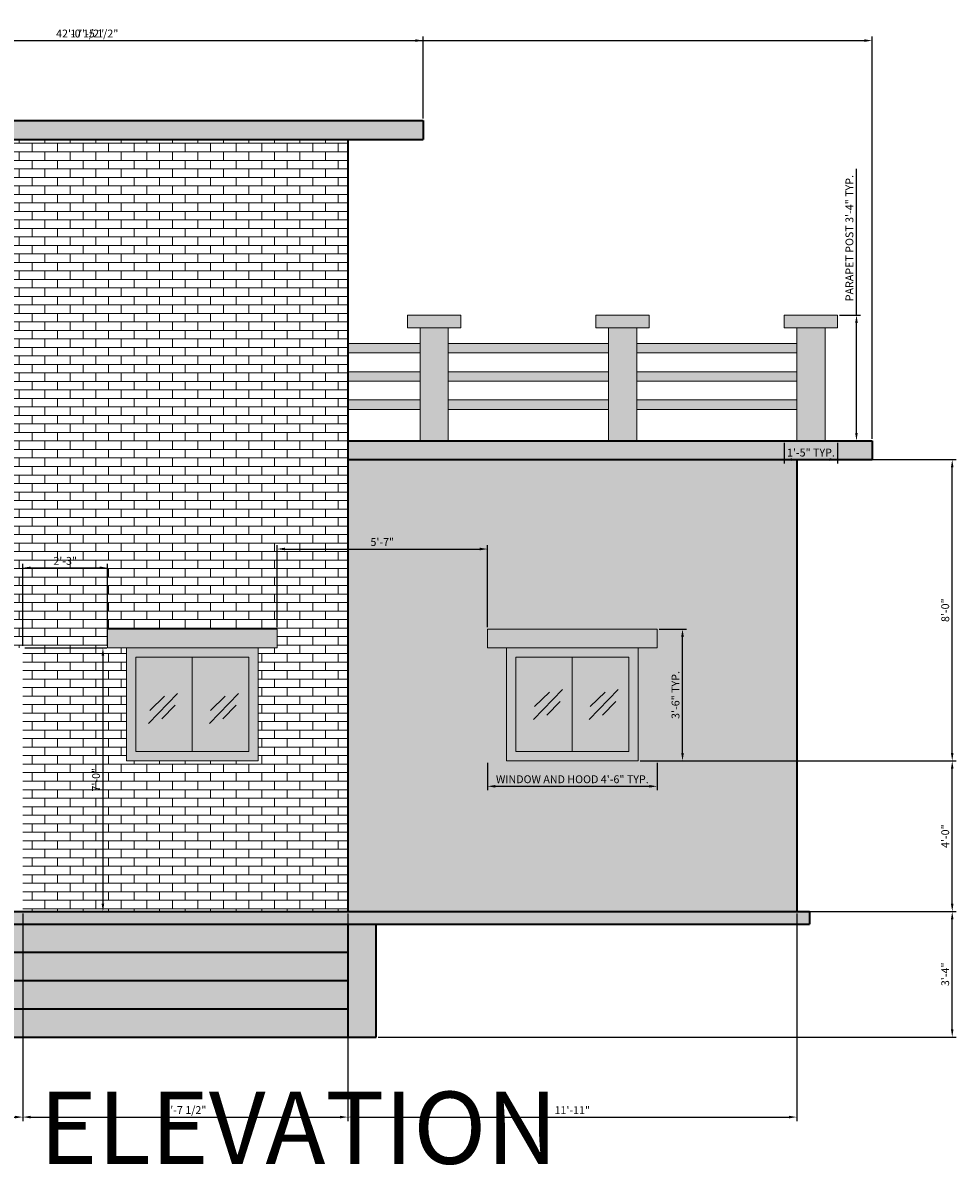
# Model space of a CAD drawing. Units: inches. Extents: x 4878 to 9282, y 5367 to 6617.
# Tile 3 of 14: x 5199 to 5496, y 5367 to 5731. Entities that reach past the tile are written whole.
import ezdxf

# ---------------------------------------------------------------- set-up
doc = ezdxf.new("R2010")
doc.units = ezdxf.units.IN
for name, color, linetype, lineweight in [('A-ANNO-DIMS', 2, 'Continuous', 18), ('A-ANNO-TITL', 3, 'Continuous', 30), ('A-ELEV', 7, 'Continuous', 35), ('A-ELEV-GLAZ', 4, 'Continuous', 20), ('A-ELEV-RAIL', 7, 'Continuous', 20), ('A-ELEV-RAIL-PATT', 7, 'Continuous', 13)]:
    doc.layers.add(name, color=color, linetype=linetype, lineweight=lineweight)
for name, color, linetype, lineweight, true_color in [('A-ELEV-BASE-PATT', 252, 'Continuous', 13, 0x939598), ('A-ELEV-CLAD-PATT', 215, 'Continuous', 13, 0xa953a0), ('A-ELEV-GLAZ-PATT', 141, 'Continuous', 13, 0xadddf7), ('A-ELEV-METL-PATT', 252, 'Continuous', 13, 0x939598), ('A-ELEV-TRIM-PATT', 11, 'Continuous', 13, 0xf27172), ('A-ELEV-WALL-PATT', 9, 'Continuous', 13, 0xafd9aa)]:
    doc.layers.add(name, color=color, linetype=linetype, lineweight=lineweight, true_color=true_color)
doc.styles.get("Standard").update_dxf_attribs({"font": 'arial.ttf'})
doc.dimstyles.new('ISO-25', dxfattribs={"dimtxt": 2.5, "dimasz": 2.5, "dimexe": 1.25, "dimexo": 0.625, "dimtad": 1, "dimdec": 0, "dimlunit": 3, "dimtxsty": 'Standard', "dimcen": 2.5, "dimadec": 0, "dimazin": 0, "dimtfac": 1, "dimtdec": 0, "dimtmove": 0, "dimatfit": 3, "dimfxl": 1, "dimarcsym": 0})

# ---------------------------------------------------------------- blocks, each defined once
blk = doc.blocks.new('PARAPET-POST-CAPPED')
for p, q in [((0, 40), (0, 36)), ((0, 40), (17, 40)), ((17, 40), (17, 36)), ((0, 36), (17, 36)), ((4, 36), (4, 0)), ((13, 36), (13, 0))]:
    blk.add_line(p, q)
blk = doc.blocks.new('WINDOW-ELEV-WITH-HOOD-36IN')
for p, q in [((0, 42), (0, 36)), ((0, 42), (54, 42)), ((54, 42), (54, 36)), ((0, 36), (54, 36)), ((6, 0), (6, 36)), ((9, 3), (9, 33)), ((9, 33), (45, 33)), ((27, 33), (27, 3)), ((45, 3), (45, 33)), ((48, 0), (48, 36)), ((6, 0), (48, 0)), ((9, 3), (45, 3))]:
    blk.add_line(p, q)
blk = doc.blocks.new('GLASS-REFLECTION-MARK')
for p, q in [((0, 0), (9.22, 9.57)), ((0.36, 4.15), (5.06, 8.67)), ((4.25, 1.44), (8.5, 5.78))]:
    blk.add_line(p, q)
blk = doc.blocks.new('*D47')
at = {"layer": 'A-ANNO-DIMS', "color": 0, "lineweight": -2, "transparency": 16777216}
for p, q in [((5464.48, 5637.76), (5464.48, 5684.38)), ((5459.1, 5637.76), (5465.73, 5637.76)), ((5464.48, 5600.26), (5464.48, 5635.26)), ((5459.1, 5597.76), (5465.73, 5597.76))]:
    blk.add_line(p, q, dxfattribs=at)
at = {"layer": 'A-ANNO-DIMS', "color": 0, "transparency": 16777216}
for points in [[(5464.06, 5635.26), (5464.89, 5635.26), (5464.48, 5637.76)], [(5464.06, 5600.26), (5464.89, 5600.26), (5464.48, 5597.76)]]:
    blk.add_solid(points, dxfattribs=at)
at = {"layer": 'Defpoints', "color": 0, "transparency": 16777216}
for p in [(5458.48, 5637.76), (5464.48, 5637.76), (5458.48, 5597.76)]:
    blk.add_point(p, dxfattribs=at)
at = {"layer": 'A-ANNO-DIMS', "color": 0, "transparency": 16777216, "insert": (5462.56, 5662.32), "char_height": 2.5, "attachment_point": 5, "rotation": 90}
blk.add_mtext('PARAPET POST 3\'-4" TYP.', dxfattribs=at)
blk = doc.blocks.new('*D48')
at = {"layer": 'A-ANNO-DIMS', "color": 0, "lineweight": -2, "transparency": 16777216}
for p, q in [((5441.48, 5597.14), (5441.48, 5590.51)), ((5458.48, 5597.14), (5458.48, 5590.51)), ((5443.98, 5591.76), (5455.98, 5591.76))]:
    blk.add_line(p, q, dxfattribs=at)
at = {"layer": 'A-ANNO-DIMS', "color": 0, "transparency": 16777216}
for points in [[(5443.98, 5592.18), (5443.98, 5591.34), (5441.48, 5591.76)], [(5455.98, 5592.18), (5455.98, 5591.34), (5458.48, 5591.76)]]:
    blk.add_solid(points, dxfattribs=at)
at = {"layer": 'Defpoints', "color": 0, "transparency": 16777216}
for p in [(5441.48, 5597.76), (5458.48, 5597.76), (5458.48, 5591.76)]:
    blk.add_point(p, dxfattribs=at)
at = {"layer": 'A-ANNO-DIMS', "color": 0, "transparency": 16777216, "insert": (5449.98, 5593.66), "char_height": 2.5, "attachment_point": 5}
blk.add_mtext('1\'-5" TYP.', dxfattribs=at)
blk = doc.blocks.new('*D51')
at = {"layer": 'A-ANNO-DIMS', "color": 0, "lineweight": -2, "transparency": 16777216}
for p, q in [((5346.98, 5495.14), (5346.98, 5486.41)), ((5400.98, 5495.14), (5400.98, 5486.41)), ((5349.48, 5487.66), (5398.48, 5487.66))]:
    blk.add_line(p, q, dxfattribs=at)
at = {"layer": 'A-ANNO-DIMS', "color": 0, "transparency": 16777216}
for points in [[(5349.48, 5488.08), (5349.48, 5487.24), (5346.98, 5487.66)], [(5398.48, 5488.08), (5398.48, 5487.24), (5400.98, 5487.66)]]:
    blk.add_solid(points, dxfattribs=at)
at = {"layer": 'Defpoints', "color": 0, "transparency": 16777216}
for p in [(5346.98, 5495.76), (5400.98, 5495.76), (5400.98, 5487.66)]:
    blk.add_point(p, dxfattribs=at)
at = {"layer": 'A-ANNO-DIMS', "color": 0, "transparency": 16777216, "insert": (5373.98, 5489.58), "char_height": 2.5, "attachment_point": 5}
blk.add_mtext('WINDOW AND HOOD 4\'-6" TYP.', dxfattribs=at)
blk = doc.blocks.new('*D52')
at = {"layer": 'A-ANNO-DIMS', "color": 0, "lineweight": -2, "transparency": 16777216}
for p, q in [((5401.6, 5537.76), (5410.33, 5537.76)), ((5409.08, 5498.26), (5409.08, 5535.26)), ((5401.6, 5495.76), (5410.33, 5495.76))]:
    blk.add_line(p, q, dxfattribs=at)
at = {"layer": 'A-ANNO-DIMS', "color": 0, "transparency": 16777216}
for points in [[(5408.66, 5535.26), (5409.49, 5535.26), (5409.08, 5537.76)], [(5408.66, 5498.26), (5409.49, 5498.26), (5409.08, 5495.76)]]:
    blk.add_solid(points, dxfattribs=at)
at = {"layer": 'Defpoints', "color": 0, "transparency": 16777216}
for p in [(5400.98, 5537.76), (5409.08, 5537.76), (5400.98, 5495.76)]:
    blk.add_point(p, dxfattribs=at)
at = {"layer": 'A-ANNO-DIMS', "color": 0, "transparency": 16777216, "insert": (5407.17, 5516.76), "char_height": 2.5, "attachment_point": 5, "rotation": 90}
blk.add_mtext('3\'-6" TYP.', dxfattribs=at)
blk = doc.blocks.new('*D88')
at = {"layer": 'A-ANNO-DIMS', "color": 0, "lineweight": -2, "transparency": 16777216}
for p, q in [((4964.98, 5598.39), (4964.98, 5726.51)), ((4967.48, 5725.26), (5466.98, 5725.26)), ((5469.48, 5598.39), (5469.48, 5726.51))]:
    blk.add_line(p, q, dxfattribs=at)
at = {"layer": 'A-ANNO-DIMS', "color": 0, "transparency": 16777216}
for points in [[(4967.48, 5725.68), (4967.48, 5724.84), (4964.98, 5725.26)], [(5466.98, 5725.68), (5466.98, 5724.84), (5469.48, 5725.26)]]:
    blk.add_solid(points, dxfattribs=at)
at = {"layer": 'Defpoints', "color": 0, "transparency": 16777216}
for p in [(5469.48, 5725.26), (4964.98, 5597.76), (5469.48, 5597.76)]:
    blk.add_point(p, dxfattribs=at)
at = {"layer": 'A-ANNO-DIMS', "color": 0, "transparency": 16777216, "insert": (5217.23, 5727.18), "char_height": 2.5, "attachment_point": 5}
blk.add_mtext('42\'-0 1/2"', dxfattribs=at)
blk = doc.blocks.new('*D92')
at = {"layer": 'A-ANNO-DIMS', "color": 0, "lineweight": -2, "transparency": 16777216}
for p, q in [((5158.98, 5447.14), (5158.98, 5381.01)), ((5198.98, 5447.14), (5198.98, 5381.01)), ((5161.48, 5382.26), (5196.48, 5382.26))]:
    blk.add_line(p, q, dxfattribs=at)
at = {"layer": 'A-ANNO-DIMS', "color": 0, "transparency": 16777216}
for points in [[(5161.48, 5382.68), (5161.48, 5381.84), (5158.98, 5382.26)], [(5196.48, 5382.68), (5196.48, 5381.84), (5198.98, 5382.26)]]:
    blk.add_solid(points, dxfattribs=at)
at = {"layer": 'Defpoints', "color": 0, "transparency": 16777216}
for p in [(5158.98, 5447.76), (5198.98, 5447.76), (5198.98, 5382.26)]:
    blk.add_point(p, dxfattribs=at)
at = {"layer": 'A-ANNO-DIMS', "color": 0, "transparency": 16777216, "insert": (5178.98, 5384.16), "char_height": 2.5, "attachment_point": 5}
blk.add_mtext('3\'-4"', dxfattribs=at)
blk = doc.blocks.new('*D93')
at = {"layer": 'A-ANNO-DIMS', "color": 0, "lineweight": -2, "transparency": 16777216}
for p, q in [((5198.98, 5447.14), (5198.98, 5381.01)), ((5302.48, 5447.14), (5302.48, 5381.01)), ((5201.48, 5382.26), (5299.98, 5382.26))]:
    blk.add_line(p, q, dxfattribs=at)
at = {"layer": 'A-ANNO-DIMS', "color": 0, "transparency": 16777216}
for points in [[(5201.48, 5382.68), (5201.48, 5381.84), (5198.98, 5382.26)], [(5299.98, 5382.68), (5299.98, 5381.84), (5302.48, 5382.26)]]:
    blk.add_solid(points, dxfattribs=at)
at = {"layer": 'Defpoints', "color": 0, "transparency": 16777216}
for p in [(5198.98, 5447.76), (5302.48, 5447.76), (5302.48, 5382.26)]:
    blk.add_point(p, dxfattribs=at)
at = {"layer": 'A-ANNO-DIMS', "color": 0, "transparency": 16777216, "insert": (5250.73, 5384.18), "char_height": 2.5, "attachment_point": 5}
blk.add_mtext('8\'-7 1/2"', dxfattribs=at)
blk = doc.blocks.new('*D94')
at = {"layer": 'A-ANNO-DIMS', "color": 0, "lineweight": -2, "transparency": 16777216}
for p, q in [((5302.48, 5447.14), (5302.48, 5381.01)), ((5445.48, 5447.14), (5445.48, 5381.01)), ((5304.98, 5382.26), (5442.98, 5382.26))]:
    blk.add_line(p, q, dxfattribs=at)
at = {"layer": 'A-ANNO-DIMS', "color": 0, "transparency": 16777216}
for points in [[(5304.98, 5382.68), (5304.98, 5381.84), (5302.48, 5382.26)], [(5442.98, 5382.68), (5442.98, 5381.84), (5445.48, 5382.26)]]:
    blk.add_solid(points, dxfattribs=at)
at = {"layer": 'Defpoints', "color": 0, "transparency": 16777216}
for p in [(5302.48, 5447.76), (5445.48, 5447.76), (5445.48, 5382.26)]:
    blk.add_point(p, dxfattribs=at)
at = {"layer": 'A-ANNO-DIMS', "color": 0, "transparency": 16777216, "insert": (5373.98, 5384.14), "char_height": 2.5, "attachment_point": 5}
blk.add_mtext('11\'-11"', dxfattribs=at)
blk = doc.blocks.new('*D95')
at = {"layer": 'A-ANNO-DIMS', "color": 0, "lineweight": -2, "transparency": 16777216}
for p, q in [((5446.1, 5591.76), (5496.23, 5591.76)), ((5494.98, 5498.26), (5494.98, 5589.26)), ((5395.6, 5495.76), (5496.23, 5495.76))]:
    blk.add_line(p, q, dxfattribs=at)
at = {"layer": 'A-ANNO-DIMS', "color": 0, "transparency": 16777216}
for points in [[(5494.56, 5589.26), (5495.39, 5589.26), (5494.98, 5591.76)], [(5494.56, 5498.26), (5495.39, 5498.26), (5494.98, 5495.76)]]:
    blk.add_solid(points, dxfattribs=at)
at = {"layer": 'Defpoints', "color": 0, "transparency": 16777216}
for p in [(5445.48, 5591.76), (5494.98, 5591.76), (5394.98, 5495.76)]:
    blk.add_point(p, dxfattribs=at)
at = {"layer": 'A-ANNO-DIMS', "color": 0, "transparency": 16777216, "insert": (5493.08, 5543.76), "char_height": 2.5, "attachment_point": 5, "rotation": 90}
blk.add_mtext('8\'-0"', dxfattribs=at)
blk = doc.blocks.new('*D96')
at = {"layer": 'A-ANNO-DIMS', "color": 0, "lineweight": -2, "transparency": 16777216}
for p, q in [((5395.6, 5495.76), (5496.23, 5495.76)), ((5494.98, 5450.26), (5494.98, 5493.26)), ((5446.1, 5447.76), (5496.23, 5447.76))]:
    blk.add_line(p, q, dxfattribs=at)
at = {"layer": 'A-ANNO-DIMS', "color": 0, "transparency": 16777216}
for points in [[(5494.56, 5493.26), (5495.39, 5493.26), (5494.98, 5495.76)], [(5494.56, 5450.26), (5495.39, 5450.26), (5494.98, 5447.76)]]:
    blk.add_solid(points, dxfattribs=at)
at = {"layer": 'Defpoints', "color": 0, "transparency": 16777216}
for p in [(5394.98, 5495.76), (5494.98, 5495.76), (5445.48, 5447.76)]:
    blk.add_point(p, dxfattribs=at)
at = {"layer": 'A-ANNO-DIMS', "color": 0, "transparency": 16777216, "insert": (5493.08, 5471.76), "char_height": 2.5, "attachment_point": 5, "rotation": 90}
blk.add_mtext('4\'-0"', dxfattribs=at)
blk = doc.blocks.new('*D98')
at = {"layer": 'A-ANNO-DIMS', "color": 0, "lineweight": -2, "transparency": 16777216}
for p, q in [((5199.6, 5531.76), (5225.73, 5531.76)), ((5224.48, 5529.26), (5224.48, 5450.26)), ((5199.6, 5447.76), (5225.73, 5447.76))]:
    blk.add_line(p, q, dxfattribs=at)
at = {"layer": 'A-ANNO-DIMS', "color": 0, "transparency": 16777216}
for points in [[(5224.06, 5529.26), (5224.89, 5529.26), (5224.48, 5531.76)], [(5224.06, 5450.26), (5224.89, 5450.26), (5224.48, 5447.76)]]:
    blk.add_solid(points, dxfattribs=at)
at = {"layer": 'Defpoints', "color": 0, "transparency": 16777216}
for p in [(5198.98, 5531.76), (5198.98, 5447.76), (5224.48, 5447.76)]:
    blk.add_point(p, dxfattribs=at)
at = {"layer": 'A-ANNO-DIMS', "color": 0, "transparency": 16777216, "insert": (5222.58, 5489.76), "char_height": 2.5, "attachment_point": 5, "rotation": 90}
blk.add_mtext('7\'-0"', dxfattribs=at)
blk = doc.blocks.new('*D117')
at = {"layer": 'A-ANNO-DIMS', "color": 0, "lineweight": -2, "transparency": 16777216}
for p, q in [((5198.98, 5532.39), (5198.98, 5558.51)), ((5225.95, 5532.39), (5225.95, 5558.51)), ((5201.48, 5557.26), (5223.45, 5557.26))]:
    blk.add_line(p, q, dxfattribs=at)
at = {"layer": 'A-ANNO-DIMS', "color": 0, "transparency": 16777216}
for points in [[(5201.48, 5557.68), (5201.48, 5556.84), (5198.98, 5557.26)], [(5223.45, 5557.68), (5223.45, 5556.84), (5225.95, 5557.26)]]:
    blk.add_solid(points, dxfattribs=at)
at = {"layer": 'Defpoints', "color": 0, "transparency": 16777216}
for p in [(5225.95, 5557.26), (5198.98, 5531.76), (5225.95, 5531.76)]:
    blk.add_point(p, dxfattribs=at)
at = {"layer": 'A-ANNO-DIMS', "color": 0, "transparency": 16777216, "insert": (5212.46, 5559.16), "char_height": 2.5, "attachment_point": 5}
blk.add_mtext('2\'-3"', dxfattribs=at)
blk = doc.blocks.new('*D118')
at = {"layer": 'A-ANNO-DIMS', "color": 0, "lineweight": -2, "transparency": 16777216}
for p, q in [((5279.95, 5538.39), (5279.95, 5564.51)), ((5282.45, 5563.26), (5344.48, 5563.26)), ((5346.98, 5538.39), (5346.98, 5564.51))]:
    blk.add_line(p, q, dxfattribs=at)
at = {"layer": 'A-ANNO-DIMS', "color": 0, "transparency": 16777216}
for points in [[(5282.45, 5563.68), (5282.45, 5562.84), (5279.95, 5563.26)], [(5344.48, 5563.68), (5344.48, 5562.84), (5346.98, 5563.26)]]:
    blk.add_solid(points, dxfattribs=at)
at = {"layer": 'Defpoints', "color": 0, "transparency": 16777216}
for p in [(5346.98, 5563.26), (5279.95, 5537.76), (5346.98, 5537.76)]:
    blk.add_point(p, dxfattribs=at)
at = {"layer": 'A-ANNO-DIMS', "color": 0, "transparency": 16777216, "insert": (5313.46, 5565.16), "char_height": 2.5, "attachment_point": 5}
blk.add_mtext('5\'-7"', dxfattribs=at)
blk = doc.blocks.new('*D119')
at = {"layer": 'A-ANNO-DIMS', "color": 0, "lineweight": -2, "transparency": 16777216}
for p, q in [((5446.1, 5447.76), (5496.23, 5447.76)), ((5494.98, 5410.26), (5494.98, 5445.26)), ((5312.1, 5407.76), (5496.23, 5407.76))]:
    blk.add_line(p, q, dxfattribs=at)
at = {"layer": 'A-ANNO-DIMS', "color": 0, "transparency": 16777216}
for points in [[(5494.56, 5445.26), (5495.39, 5445.26), (5494.98, 5447.76)], [(5494.56, 5410.26), (5495.39, 5410.26), (5494.98, 5407.76)]]:
    blk.add_solid(points, dxfattribs=at)
at = {"layer": 'Defpoints', "color": 0, "transparency": 16777216}
for p in [(5445.48, 5447.76), (5494.98, 5447.76), (5311.48, 5407.76)]:
    blk.add_point(p, dxfattribs=at)
at = {"layer": 'A-ANNO-DIMS', "color": 0, "transparency": 16777216, "insert": (5493.07, 5427.76), "char_height": 2.5, "attachment_point": 5, "rotation": 90}
blk.add_mtext('3\'-4"', dxfattribs=at)
blk = doc.blocks.new('*D120')
at = {"layer": 'A-ANNO-DIMS', "color": 0, "lineweight": -2, "transparency": 16777216}
for p, q in [((5116.98, 5700.39), (5116.98, 5726.51)), ((5119.48, 5725.26), (5323.98, 5725.26)), ((5326.48, 5700.39), (5326.48, 5726.51))]:
    blk.add_line(p, q, dxfattribs=at)
at = {"layer": 'A-ANNO-DIMS', "color": 0, "transparency": 16777216}
for points in [[(5119.48, 5725.68), (5119.48, 5724.84), (5116.98, 5725.26)], [(5323.98, 5725.68), (5323.98, 5724.84), (5326.48, 5725.26)]]:
    blk.add_solid(points, dxfattribs=at)
at = {"layer": 'Defpoints', "color": 0, "transparency": 16777216}
for p in [(5326.48, 5725.26), (5116.98, 5699.76), (5326.48, 5699.76)]:
    blk.add_point(p, dxfattribs=at)
at = {"layer": 'A-ANNO-DIMS', "color": 0, "transparency": 16777216, "insert": (5221.73, 5727.18), "char_height": 2.5, "attachment_point": 5}
blk.add_mtext('17\'-5 1/2"', dxfattribs=at)

msp = doc.modelspace()

# ---------------------------------------------------------------- hatches: boundary and pattern name
at = {"layer": 'A-ELEV-BASE-PATT'}
h = msp.add_hatch(color=256, dxfattribs=at)
h.dxf.hatch_style = 1
h.paths.add_polyline_path([(4984.98, 5447.76), (4984.98, 5443.76), (5449.48, 5443.76), (5449.48, 5447.76)])
h = msp.add_hatch(color=256, dxfattribs=at)
h.dxf.hatch_style = 1
h.paths.add_polyline_path([(5140.98, 5443.76), (5131.98, 5443.76), (5131.98, 5407.76), (5140.98, 5407.76)])
h.paths.add_polyline_path([(5302.48, 5407.76), (5311.48, 5407.76), (5311.48, 5443.76), (5302.48, 5443.76)])
h = msp.add_hatch(color=256, dxfattribs=at)
h.dxf.hatch_style = 1
h.paths.add_polyline_path([(5302.48, 5434.76), (5302.48, 5443.76), (5140.98, 5443.76), (5140.98, 5434.76)])
h.paths.add_polyline_path([(5302.48, 5416.76), (5302.48, 5425.76), (5140.98, 5425.76), (5140.98, 5416.76)])
h = msp.add_hatch(color=256, dxfattribs=at)
h.dxf.hatch_style = 1
h.paths.add_polyline_path([(5302.48, 5407.76), (5302.48, 5416.76), (5140.98, 5416.76), (5140.98, 5407.76)])
h.paths.add_polyline_path([(5140.98, 5434.76), (5140.98, 5425.76), (5302.48, 5425.76), (5302.48, 5434.76)])
at = {"layer": 'A-ELEV-CLAD-PATT'}
h = msp.add_hatch(dxfattribs=at)
h.set_pattern_fill('AR-BRSTD', color=256, scale=0.04)
h.set_pattern_definition([(0, (-2235.2307, 189.171), (0, 2.709672), []), (90, (-2235.2307, 189.171), (-4.064, 2.709672), [2.709672, -2.709672])])
h.paths.add_polyline_path([(5140.98, 5447.76), (5158.98, 5447.76), (5158.98, 5531.76), (5198.98, 5531.76), (5198.98, 5447.76), (5302.48, 5447.76), (5302.48, 5693.76), (5140.98, 5693.76)])
h.paths.add_polyline_path([(5225.95, 5537.76), (5279.95, 5537.76), (5279.95, 5531.76), (5273.95, 5531.76), (5273.95, 5495.76), (5231.95, 5495.76), (5231.95, 5531.76), (5225.95, 5531.76)], flags=16)
h.paths.add_polyline_path([(5234.95, 5528.76), (5270.95, 5528.76), (5270.95, 5498.76), (5234.95, 5498.76)], flags=0)
at = {"layer": 'A-ELEV-GLAZ-PATT'}
h = msp.add_hatch(color=256, dxfattribs=at)
h.dxf.hatch_style = 1
h.paths.add_polyline_path([(5252.95, 5528.76), (5234.95, 5528.76), (5234.95, 5498.76), (5252.95, 5498.76)])
h.paths.add_polyline_path([(5270.95, 5528.76), (5252.95, 5528.76), (5252.95, 5498.76), (5270.95, 5498.76)])
h.paths.add_polyline_path([(5373.98, 5528.76), (5355.98, 5528.76), (5355.98, 5498.76), (5373.98, 5498.76)])
h.paths.add_polyline_path([(5391.98, 5528.76), (5373.98, 5528.76), (5373.98, 5498.76), (5391.98, 5498.76)])
at = {"layer": 'A-ELEV-METL-PATT'}
h = msp.add_hatch(color=256, dxfattribs=at)
h.dxf.hatch_style = 1
h.paths.add_polyline_path([(5231.95, 5495.76), (5273.95, 5495.76), (5273.95, 5531.76), (5231.95, 5531.76)])
h.paths.add_polyline_path([(5234.95, 5528.76), (5270.95, 5528.76), (5270.95, 5498.76), (5234.95, 5498.76)], flags=16)
h.paths.add_polyline_path([(5352.98, 5495.76), (5394.98, 5495.76), (5394.98, 5531.76), (5352.98, 5531.76)])
h.paths.add_polyline_path([(5355.98, 5528.76), (5391.98, 5528.76), (5391.98, 5498.76), (5355.98, 5498.76)], flags=16)
at = {"layer": 'A-ELEV-RAIL-PATT'}
h = msp.add_hatch(color=256, dxfattribs=at)
h.dxf.hatch_style = 1
h.paths.add_polyline_path([(5048.98, 5633.76), (5039.98, 5633.76), (5039.98, 5597.76), (5048.98, 5597.76)])
h.paths.add_polyline_path([(5108.98, 5633.76), (5099.98, 5633.76), (5099.98, 5597.76), (5108.98, 5597.76)])
h.paths.add_polyline_path([(4988.98, 5633.76), (4979.98, 5633.76), (4979.98, 5597.76), (4988.98, 5597.76)])
h.paths.add_polyline_path([(5334.48, 5633.76), (5325.48, 5633.76), (5325.48, 5597.76), (5334.48, 5597.76)])
h.paths.add_polyline_path([(5385.48, 5597.76), (5394.48, 5597.76), (5394.48, 5633.76), (5385.48, 5633.76)])
h.paths.add_polyline_path([(5445.48, 5597.76), (5454.48, 5597.76), (5454.48, 5633.76), (5445.48, 5633.76)])
h = msp.add_hatch(color=256, dxfattribs=at)
h.dxf.hatch_style = 1
h.paths.add_polyline_path([(5039.98, 5628.76), (4988.98, 5628.76), (4988.98, 5625.76), (5039.98, 5625.76)])
h.paths.add_polyline_path([(5099.98, 5628.76), (5048.98, 5628.76), (5048.98, 5625.76), (5099.98, 5625.76)])
h.paths.add_polyline_path([(5099.98, 5619.76), (5048.98, 5619.76), (5048.98, 5616.76), (5099.98, 5616.76)])
h.paths.add_polyline_path([(5099.98, 5610.76), (5048.98, 5610.76), (5048.98, 5607.76), (5099.98, 5607.76)])
h.paths.add_polyline_path([(5140.98, 5628.76), (5108.98, 5628.76), (5108.98, 5625.76), (5140.98, 5625.76)])
h.paths.add_polyline_path([(5140.98, 5619.76), (5108.98, 5619.76), (5108.98, 5616.76), (5140.98, 5616.76)])
h.paths.add_polyline_path([(5140.98, 5610.76), (5108.98, 5610.76), (5108.98, 5607.76), (5140.98, 5607.76)])
h.paths.add_polyline_path([(5325.48, 5610.76), (5302.48, 5610.76), (5302.48, 5607.76), (5325.48, 5607.76)])
h.paths.add_polyline_path([(5325.48, 5619.76), (5302.48, 5619.76), (5302.48, 5616.76), (5325.48, 5616.76)])
h.paths.add_polyline_path([(5325.48, 5628.76), (5302.48, 5628.76), (5302.48, 5625.76), (5325.48, 5625.76)])
h.paths.add_polyline_path([(5385.48, 5628.76), (5334.48, 5628.76), (5334.48, 5625.76), (5385.48, 5625.76)])
h.paths.add_polyline_path([(5385.48, 5619.76), (5334.48, 5619.76), (5334.48, 5616.76), (5385.48, 5616.76)])
h.paths.add_polyline_path([(5385.48, 5610.76), (5334.48, 5610.76), (5334.48, 5607.76), (5385.48, 5607.76)])
h.paths.add_polyline_path([(5445.48, 5628.76), (5394.48, 5628.76), (5394.48, 5625.76), (5445.48, 5625.76)])
h.paths.add_polyline_path([(5445.48, 5619.76), (5394.48, 5619.76), (5394.48, 5616.76), (5445.48, 5616.76)])
h.paths.add_polyline_path([(5445.48, 5610.76), (5394.48, 5610.76), (5394.48, 5607.76), (5445.48, 5607.76)])
at = {"layer": 'A-ELEV-TRIM-PATT'}
h = msp.add_hatch(color=256, dxfattribs=at)
h.dxf.hatch_style = 1
h.paths.add_polyline_path([(5140.98, 5591.76), (5140.98, 5597.76), (4964.98, 5597.76), (4964.98, 5591.76)])
h.paths.add_polyline_path([(5112.98, 5633.76), (5112.98, 5637.76), (5095.98, 5637.76), (5095.98, 5633.76)])
h.paths.add_polyline_path([(5035.98, 5637.76), (5035.98, 5633.76), (5052.98, 5633.76), (5052.98, 5637.76)])
h.paths.add_polyline_path([(4975.98, 5637.76), (4975.98, 5633.76), (4992.98, 5633.76), (4992.98, 5637.76)])
h.paths.add_polyline_path([(5116.98, 5699.76), (5116.98, 5693.76), (5326.48, 5693.76), (5326.48, 5699.76)])
h.paths.add_polyline_path([(5321.48, 5637.76), (5321.48, 5633.76), (5338.48, 5633.76), (5338.48, 5637.76)])
h.paths.add_polyline_path([(5381.48, 5637.76), (5381.48, 5633.76), (5398.48, 5633.76), (5398.48, 5637.76)])
h.paths.add_polyline_path([(5441.48, 5637.76), (5441.48, 5633.76), (5458.48, 5633.76), (5458.48, 5637.76)])
h.paths.add_polyline_path([(5469.48, 5591.76), (5469.48, 5597.76), (5302.48, 5597.76), (5302.48, 5591.76)])
h.paths.add_polyline_path([(5346.98, 5537.76), (5346.98, 5531.76), (5400.98, 5531.76), (5400.98, 5537.76)])
h.paths.add_polyline_path([(5279.95, 5531.76), (5279.95, 5537.76), (5225.95, 5537.76), (5225.95, 5531.76)])
at = {"layer": 'A-ELEV-WALL-PATT'}
h = msp.add_hatch(color=256, dxfattribs=at)
h.dxf.hatch_style = 1
h.paths.add_polyline_path([(5302.48, 5591.76), (5302.48, 5447.76), (5445.48, 5447.76), (5445.48, 5591.76)])
h.paths.add_polyline_path([(5400.98, 5537.76), (5400.98, 5531.76), (5394.98, 5531.76), (5394.98, 5495.76), (5352.98, 5495.76), (5352.98, 5531.76), (5346.98, 5531.76), (5346.98, 5537.76)], flags=16)
h.paths.add_polyline_path([(5391.98, 5528.76), (5391.98, 5498.76), (5355.98, 5498.76), (5355.98, 5528.76)], flags=0)

# ---------------------------------------------------------------- linework, layer by layer
at = {"layer": 'A-ELEV'}
for p, q in [((5116.98, 5699.76), (5326.48, 5699.76)), ((5326.48, 5699.76), (5326.48, 5693.76)), ((5116.98, 5693.76), (5326.48, 5693.76)), ((5302.48, 5693.76), (5302.48, 5447.76)), ((5302.48, 5597.76), (5469.48, 5597.76)), ((5469.48, 5597.76), (5469.48, 5591.76)), ((5302.48, 5591.76), (5469.48, 5591.76)), ((5445.48, 5591.76), (5445.48, 5447.76)), ((4984.98, 5447.76), (5449.48, 5447.76)), ((5449.48, 5447.76), (5449.48, 5443.76)), ((4984.98, 5443.76), (5449.48, 5443.76)), ((5302.48, 5443.76), (5302.48, 5407.76)), ((5311.48, 5407.76), (5311.48, 5443.76)), ((5140.98, 5434.76), (5302.48, 5434.76)), ((5140.98, 5425.76), (5302.48, 5425.76)), ((5140.98, 5416.76), (5302.48, 5416.76)), ((5131.98, 5407.76), (5311.48, 5407.76))]:
    msp.add_line(p, q, dxfattribs=at)
at = {"layer": 'A-ELEV-RAIL'}
for p, q in [((5302.48, 5628.76), (5325.48, 5628.76)), ((5334.48, 5628.76), (5385.48, 5628.76)), ((5394.48, 5628.76), (5445.48, 5628.76)), ((5302.48, 5625.76), (5325.48, 5625.76)), ((5334.48, 5625.76), (5385.48, 5625.76)), ((5394.48, 5625.76), (5445.48, 5625.76)), ((5302.48, 5619.76), (5325.48, 5619.76)), ((5334.48, 5619.76), (5385.48, 5619.76)), ((5394.48, 5619.76), (5445.48, 5619.76)), ((5302.48, 5616.76), (5325.48, 5616.76)), ((5334.48, 5616.76), (5385.48, 5616.76)), ((5394.48, 5616.76), (5445.48, 5616.76)), ((5302.48, 5610.76), (5325.48, 5610.76)), ((5334.48, 5610.76), (5385.48, 5610.76)), ((5394.48, 5610.76), (5445.48, 5610.76)), ((5302.48, 5607.76), (5325.48, 5607.76)), ((5334.48, 5607.76), (5385.48, 5607.76)), ((5394.48, 5607.76), (5445.48, 5607.76))]:
    msp.add_line(p, q, dxfattribs=at)

# ---------------------------------------------------------------- block references
at = {"layer": 'A-ELEV-GLAZ'}
for name, p in [('WINDOW-ELEV-WITH-HOOD-36IN', (5225.95, 5495.76)), ('WINDOW-ELEV-WITH-HOOD-36IN', (5346.98, 5495.76)), ('GLASS-REFLECTION-MARK', (5361.6, 5508.93)), ('GLASS-REFLECTION-MARK', (5379.35, 5508.93)), ('GLASS-REFLECTION-MARK', (5239.03, 5507.69)), ('GLASS-REFLECTION-MARK', (5258.39, 5507.69))]:
    msp.add_blockref(name, p, dxfattribs=at)
at = {"layer": 'A-ELEV-RAIL'}
for p in [(5321.48, 5597.76), (5381.48, 5597.76), (5441.48, 5597.76)]:
    msp.add_blockref('PARAPET-POST-CAPPED', p, dxfattribs=at)

# ---------------------------------------------------------------- texts
at = {"layer": 'A-ANNO-TITL', "insert": (5095.17, 5390.36), "char_height": 23, "attachment_point": 1}
msp.add_mtext_dynamic_manual_height_columns('FRONT ELEVATION', width=1356.1732, gutter_width=12.5, heights=[0], dxfattribs=at)

# ---------------------------------------------------------------- dimensions: what is measured, and where the dimension line sits
at = {"layer": 'A-ANNO-DIMS'}
for base, p1, p2, picture, middle in [((5469.48, 5725.26), (4964.98, 5597.76), (5469.48, 5597.76), '*D88', (5217.23, 5727.18)), ((5326.48, 5725.26), (5116.98, 5699.76), (5326.48, 5699.76), '*D120', (5221.73, 5727.18)), ((5346.98, 5563.26), (5279.95, 5537.76), (5346.98, 5537.76), '*D118', (5313.46, 5565.16)), ((5225.95, 5557.26), (5198.98, 5531.76), (5225.95, 5531.76), '*D117', (5212.46, 5559.16)), ((5198.98, 5382.26), (5158.98, 5447.76), (5198.98, 5447.76), '*D92', (5178.98, 5384.16)), ((5302.48, 5382.26), (5198.98, 5447.76), (5302.48, 5447.76), '*D93', (5250.73, 5384.18)), ((5445.48, 5382.26), (5302.48, 5447.76), (5445.48, 5447.76), '*D94', (5373.98, 5384.14))]:
    dim = msp.add_linear_dim(base=base, p1=p1, p2=p2, dimstyle='ISO-25', override={"dimdec": 1, "dimlfac": 1, "dimrnd": 0, "dimzin": 1, "dimdsep": 46, "dimlunit": 4, "dimfrac": 2}, dxfattribs=at)
    dim.commit()
    dim.dimension.update_dxf_attribs({"geometry": picture, "text_midpoint": middle})
for base, p1, p2, text, picture, middle in [((5464.48, 5637.76), (5458.48, 5597.76), (5458.48, 5637.76), 'PARAPET POST <> TYP.', '*D47', (5462.56, 5662.32)), ((5409.08, 5537.76), (5400.98, 5495.76), (5400.98, 5537.76), '<> TYP.', '*D52', (5407.17, 5516.76))]:
    dim = msp.add_linear_dim(base=base, p1=p1, p2=p2, angle=90, text=text, dimstyle='ISO-25', override={"dimdec": 1, "dimlfac": 1, "dimrnd": 0, "dimzin": 1, "dimdsep": 46, "dimlunit": 4, "dimfrac": 2}, dxfattribs=at)
    dim.commit()
    dim.dimension.update_dxf_attribs({"geometry": picture, "text_midpoint": middle})
for base, p1, p2, text, picture, middle in [((5458.48, 5591.76), (5441.48, 5597.76), (5458.48, 5597.76), '<> TYP.', '*D48', (5449.98, 5593.66)), ((5400.98, 5487.66), (5346.98, 5495.76), (5400.98, 5495.76), 'WINDOW AND HOOD <> TYP.', '*D51', (5373.98, 5489.58))]:
    dim = msp.add_linear_dim(base=base, p1=p1, p2=p2, text=text, dimstyle='ISO-25', override={"dimdec": 1, "dimlfac": 1, "dimrnd": 0, "dimzin": 1, "dimdsep": 46, "dimlunit": 4, "dimfrac": 2}, dxfattribs=at)
    dim.commit()
    dim.dimension.update_dxf_attribs({"geometry": picture, "text_midpoint": middle})
for base, p1, p2, angle, picture, middle in [((5494.98, 5591.76), (5394.98, 5495.76), (5445.48, 5591.76), 90, '*D95', (5493.08, 5543.76)), ((5224.48, 5447.76), (5198.98, 5531.76), (5198.98, 5447.76), 270, '*D98', (5222.58, 5489.76)), ((5494.98, 5495.76), (5445.48, 5447.76), (5394.98, 5495.76), 90, '*D96', (5493.08, 5471.76)), ((5494.98, 5447.76), (5311.48, 5407.76), (5445.48, 5447.76), 90, '*D119', (5493.07, 5427.76))]:
    dim = msp.add_linear_dim(base=base, p1=p1, p2=p2, angle=angle, dimstyle='ISO-25', override={"dimdec": 1, "dimlfac": 1, "dimrnd": 0, "dimzin": 1, "dimdsep": 46, "dimlunit": 4, "dimfrac": 2}, dxfattribs=at)
    dim.commit()
    dim.dimension.update_dxf_attribs({"geometry": picture, "text_midpoint": middle})

doc.saveas('drawing.dxf')
